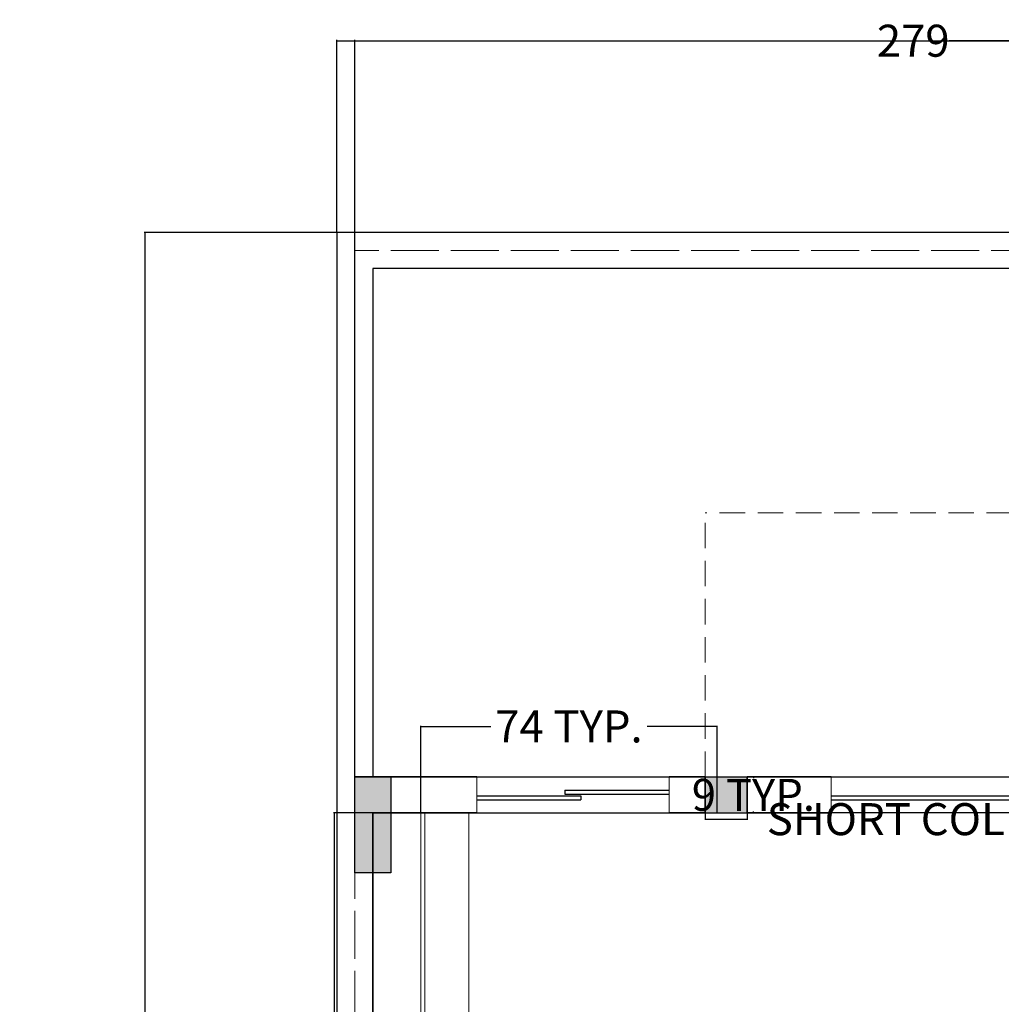
# Model space of a CAD drawing. Units: inches. Extents: x -48 to 50072, y 0 to 21068.
# Tile 67 of 75: x 680 to 925, y 1049 to 1295. Entities that reach past the tile are written whole.
import ezdxf

# ---------------------------------------------------------------- set-up
doc = ezdxf.new("R2010")
doc.units = ezdxf.units.IN
doc.header["$MEASUREMENT"] = 0
doc.linetypes.add('ACAD_ISO02W100', pattern=[15, 12, -3])
doc.linetypes.add('HIDDEN', pattern=[9.525, 6.35, -3.175])
for name, color, linetype, lineweight in [('A-ANNO-DIMS', 2, 'Continuous', 18), ('A-COLS', 1, 'Continuous', 35), ('A-DOOR', 4, 'Continuous', 18), ('A-FLOR-CASE', 9, 'Continuous', 18), ('A-FLOR-OVHD', 8, 'HIDDEN', 13), ('A-GLAZ', 4, 'Continuous', 18), ('A-WALL', 7, 'Continuous', 35), ('C-PROP', 7, 'Continuous', 25), ('C-PROP-REF', 32, 'ACAD_ISO02W100', 13)]:
    doc.layers.add(name, color=color, linetype=linetype, lineweight=lineweight)
doc.layers.add('Layer3', color=176, linetype='Continuous')
doc.styles.get("Standard").update_dxf_attribs({"font": 'arial.ttf'})
doc.dimstyles.get("Standard").update_dxf_attribs({"dimtxt": 8, "dimasz": 0.18, "dimexe": 0.18, "dimexo": 0.0625, "dimgap": 0.09, "dimtad": 0, "dimtih": 1, "dimtoh": 1, "dimdec": 1, "dimzin": 0, "dimdsep": 46, "dimlunit": 4, "dimtxsty": 'Standard', "dimblk": 'ARCHTICK', "dimcen": 0.09, "dimadec": 0, "dimazin": 0, "dimtfac": 1, "dimtdec": 1, "dimtofl": 0, "dimtmove": 0, "dimatfit": 3, "dimldrblk": 'ARCHTICK', "dimfxl": 1, "dimtolj": 1, "dimtzin": 0, "dimarcsym": 0})

# ---------------------------------------------------------------- blocks, each defined once
blk = doc.blocks.new('khll')
at = {"layer": 'Defpoints'}
h = blk.add_hatch(color=256, dxfattribs=at)
h.dxf.hatch_style = 1
h.paths.add_polyline_path([(105.52, 1025.77), (116.02, 1025.77), (116.02, 1034.77), (105.52, 1034.77)])
for p, q in [((105.52, 1025.77), (105.52, 1034.77)), ((116.02, 1025.77), (116.02, 1034.77))]:
    blk.add_line(p, q)
for p, q in [((105.52, 1034.77), (116.02, 1034.77)), ((105.52, 1025.77), (116.02, 1025.77))]:
    blk.add_line(p, q, dxfattribs=at)
blk = doc.blocks.new('bnniku')
at = {"layer": 'Defpoints'}
h = blk.add_hatch(color=256, dxfattribs=at)
h.dxf.hatch_style = 1
h.paths.add_polyline_path([(767.55, 1114.04), (758.55, 1114.04), (758.55, 1090.04), (767.55, 1090.04)])
for p, q in [((758.55, 1114.04), (767.55, 1114.04)), ((758.55, 1090.04), (758.55, 1114.04)), ((767.55, 1114.04), (767.55, 1090.04)), ((767.55, 1090.04), (758.55, 1090.04))]:
    blk.add_line(p, q, dxfattribs=at)
blk = doc.blocks.new('windom')
for p, q in [((48.52, 1025.77), (48.52, 1034.77)), ((96.52, 1025.77), (96.52, 1034.77))]:
    blk.add_line(p, q)
at = {"layer": 'Defpoints'}
for p, q in [((70.52, 1031.47), (96.52, 1031.47)), ((70.52, 1031.47), (70.52, 1030.47)), ((48.52, 1030.07), (74.52, 1030.07)), ((48.52, 1029.07), (74.52, 1029.07)), ((70.52, 1030.47), (96.52, 1030.47)), ((74.52, 1030.07), (74.52, 1029.07))]:
    blk.add_line(p, q, dxfattribs=at)
at = {"layer": 'Layer3'}
for p, q in [((48.52, 1034.77), (96.52, 1034.77)), ((48.52, 1025.77), (96.52, 1025.77))]:
    blk.add_line(p, q, dxfattribs=at)
blk = doc.blocks.new('sliding')
blk.add_line((137.02, 1025.77), (137.02, 1034.77))
at = {"layer": 'Defpoints'}
for p, q in [((234.12, 1034.77), (234.12, 1025.77)), ((183.57, 1031.47), (234.12, 1031.47)), ((183.57, 1031.47), (183.57, 1030.47)), ((137.02, 1030.07), (187.57, 1030.07)), ((137.02, 1029.07), (187.57, 1029.07)), ((183.57, 1030.47), (234.12, 1030.47)), ((187.57, 1030.07), (187.57, 1029.07))]:
    blk.add_line(p, q, dxfattribs=at)
at = {"layer": 'Layer3'}
for p, q in [((137.02, 1034.77), (234.12, 1034.77)), ((234.12, 1025.77), (137.02, 1025.77))]:
    blk.add_line(p, q, dxfattribs=at)
blk = doc.blocks.new('WARDROBE-L-RETURN')
for p, q in [((0, 144), (0, 0)), ((1, 144), (1, 1)), ((12, 144), (12, 12)), ((74, 12), (12, 12)), ((74, 1), (1, 1)), ((74, 0), (0, 0))]:
    blk.add_line(p, q)
blk = doc.blocks.new('_ArchTick')
at = {"color": 0, "linetype": 'ByBlock', "const_width": 0.15}
blk.add_lwpolyline([(-0.5, -0.5), (0.5, 0.5)], dxfattribs=at)
blk = doc.blocks.new('*D50')
at = {"layer": 'A-ANNO-DIMS', "color": 0, "lineweight": -2, "transparency": 16777216}
for p, q in [((850.76, 1096.4), (850.76, 1094.71)), ((850.76, 1094.89), (861.26, 1094.89)), ((861.26, 1096.4), (861.26, 1094.71)), ((861.26, 1094.89), (861.44, 1094.89))]:
    blk.add_line(p, q, dxfattribs=at)
at = {"layer": 'Defpoints', "color": 0, "transparency": 16777216}
for p in [(850.76, 1096.46), (861.26, 1096.46), (861.26, 1094.89)]:
    blk.add_point(p, dxfattribs=at)
at = {"layer": 'A-ANNO-DIMS', "color": 0, "lineweight": -2, "transparency": 16777216, "xscale": 0.18, "yscale": 0.18, "zscale": 0.18, "rotation": 180}
blk.add_blockref('_ArchTick', (850.76, 1094.89), dxfattribs=at)
at = {"layer": 'A-ANNO-DIMS', "color": 0, "lineweight": -2, "transparency": 16777216, "xscale": 0.18, "yscale": 0.18, "zscale": 0.18}
blk.add_blockref('_ArchTick', (861.26, 1094.89), dxfattribs=at)
at = {"layer": 'A-ANNO-DIMS', "color": 0, "transparency": 16777216, "insert": (927.86, 1094.89), "char_height": 8, "attachment_point": 5}
blk.add_mtext('\\A1;SHORT COLUMN 11 TYP.', dxfattribs=at)
blk = doc.blocks.new('*D51')
at = {"layer": 'A-ANNO-DIMS', "color": 0, "lineweight": -2, "transparency": 16777216}
for p, q in [((861.32, 1105.46), (863.02, 1105.46)), ((862.84, 1105.46), (862.84, 1105.14)), ((861.32, 1096.46), (863.02, 1096.46)), ((862.84, 1096.46), (862.84, 1096.79))]:
    blk.add_line(p, q, dxfattribs=at)
at = {"layer": 'Defpoints', "color": 0, "transparency": 16777216}
for p in [(861.26, 1105.46), (862.84, 1105.46), (861.26, 1096.46)]:
    blk.add_point(p, dxfattribs=at)
at = {"layer": 'A-ANNO-DIMS', "color": 0, "lineweight": -2, "transparency": 16777216, "xscale": 0.18, "yscale": 0.18, "zscale": 0.18}
for p, rotation in [((862.84, 1105.46), 90), ((862.84, 1096.46), 270)]:
    blk.add_blockref('_ArchTick', p, dxfattribs=dict(at, rotation=rotation))
at = {"layer": 'A-ANNO-DIMS', "color": 0, "transparency": 16777216, "insert": (862.84, 1100.96), "char_height": 8, "attachment_point": 5}
blk.add_mtext('\\A1;9 TYP.', dxfattribs=at)
blk = doc.blocks.new('*D102')
at = {"layer": 'A-ANNO-DIMS', "color": 0, "lineweight": -2, "transparency": 16777216}
for p, q in [((779.7, 1096.46), (757.98, 1096.46)), ((758.16, 1096.46), (758.16, 1028.69)), ((758.16, 952.46), (758.16, 1020.23)), ((779.7, 952.46), (757.98, 952.46))]:
    blk.add_line(p, q, dxfattribs=at)
at = {"layer": 'Defpoints', "color": 0, "transparency": 16777216}
for p in [(758.16, 1096.46), (779.76, 1096.46), (779.76, 952.46)]:
    blk.add_point(p, dxfattribs=at)
at = {"layer": 'A-ANNO-DIMS', "color": 0, "lineweight": -2, "transparency": 16777216, "xscale": 0.18, "yscale": 0.18, "zscale": 0.18}
for p, rotation in [((758.16, 1096.46), 90), ((758.16, 952.46), 270)]:
    blk.add_blockref('_ArchTick', p, dxfattribs=dict(at, rotation=rotation))
at = {"layer": 'A-ANNO-DIMS', "color": 0, "transparency": 16777216, "insert": (758.16, 1024.46), "char_height": 8, "attachment_point": 5}
blk.add_mtext('\\A1;L-RETURN WARDROBE 144 TYP.', dxfattribs=at)
blk = doc.blocks.new('*D103')
at = {"layer": 'A-ANNO-DIMS', "color": 0, "lineweight": -2, "transparency": 16777216}
for p, q in [((779.76, 1096.53), (779.76, 1118.24)), ((779.76, 1118.06), (797.23, 1118.06)), ((853.76, 1118.06), (836.29, 1118.06)), ((853.76, 1096.53), (853.76, 1118.24))]:
    blk.add_line(p, q, dxfattribs=at)
at = {"layer": 'Defpoints', "color": 0, "transparency": 16777216}
for p in [(853.76, 1118.06), (779.76, 1096.46), (853.76, 1096.46)]:
    blk.add_point(p, dxfattribs=at)
at = {"layer": 'A-ANNO-DIMS', "color": 0, "lineweight": -2, "transparency": 16777216, "xscale": 0.18, "yscale": 0.18, "zscale": 0.18, "rotation": 180}
blk.add_blockref('_ArchTick', (779.76, 1118.06), dxfattribs=at)
at = {"layer": 'A-ANNO-DIMS', "color": 0, "lineweight": -2, "transparency": 16777216, "xscale": 0.18, "yscale": 0.18, "zscale": 0.18}
blk.add_blockref('_ArchTick', (853.76, 1118.06), dxfattribs=at)
at = {"layer": 'A-ANNO-DIMS', "color": 0, "transparency": 16777216, "insert": (816.76, 1118.06), "char_height": 8, "attachment_point": 5}
blk.add_mtext('\\A1;74 TYP.', dxfattribs=at)
blk = doc.blocks.new('*D129')
at = {"layer": 'A-ANNO-DIMS', "color": 0, "lineweight": -2, "transparency": 16777216}
for p, q in [((758.76, 1241.53), (758.76, 1289.59)), ((758.76, 1289.41), (1019.85, 1289.41)), ((1298.76, 1289.41), (1037.67, 1289.41)), ((1298.76, 1241.53), (1298.76, 1289.59))]:
    blk.add_line(p, q, dxfattribs=at)
at = {"layer": 'Defpoints', "color": 0, "transparency": 16777216}
for p in [(1298.76, 1289.41), (758.76, 1241.46), (1298.76, 1241.46)]:
    blk.add_point(p, dxfattribs=at)
at = {"layer": 'A-ANNO-DIMS', "color": 0, "lineweight": -2, "transparency": 16777216, "xscale": 0.18, "yscale": 0.18, "zscale": 0.18, "rotation": 180}
blk.add_blockref('_ArchTick', (758.76, 1289.41), dxfattribs=at)
at = {"layer": 'A-ANNO-DIMS', "color": 0, "lineweight": -2, "transparency": 16777216, "xscale": 0.18, "yscale": 0.18, "zscale": 0.18}
blk.add_blockref('_ArchTick', (1298.76, 1289.41), dxfattribs=at)
at = {"layer": 'A-ANNO-DIMS', "color": 0, "transparency": 16777216, "insert": (1028.76, 1289.41), "char_height": 8, "attachment_point": 5}
blk.add_mtext('\\A1;540', dxfattribs=at)
blk = doc.blocks.new('*D130')
at = {"layer": 'A-ANNO-DIMS', "color": 0, "lineweight": -2, "transparency": 16777216}
for p, q in [((758.7, 1241.46), (710.63, 1241.46)), ((710.81, 1241.46), (710.81, 767.29)), ((710.81, 284.76), (710.81, 758.94)), ((758.7, 284.76), (710.63, 284.76))]:
    blk.add_line(p, q, dxfattribs=at)
at = {"layer": 'Defpoints', "color": 0, "transparency": 16777216}
for p in [(710.81, 1241.46), (758.76, 1241.46), (758.76, 284.76)]:
    blk.add_point(p, dxfattribs=at)
at = {"layer": 'A-ANNO-DIMS', "color": 0, "lineweight": -2, "transparency": 16777216, "xscale": 0.18, "yscale": 0.18, "zscale": 0.18}
for p, rotation in [((710.81, 1241.46), 90), ((710.81, 284.76), 270)]:
    blk.add_blockref('_ArchTick', p, dxfattribs=dict(at, rotation=rotation))
at = {"layer": 'A-ANNO-DIMS', "color": 0, "transparency": 16777216, "insert": (710.81, 763.11), "char_height": 8, "attachment_point": 5}
blk.add_mtext('\\A1;956.7', dxfattribs=at)
blk = doc.blocks.new('*D142')
at = {"layer": 'A-ANNO-DIMS', "color": 0, "lineweight": -2, "transparency": 16777216}
for p, q in [((763.26, 1105.53), (763.26, 1289.59)), ((763.26, 1289.41), (893.76, 1289.41)), ((1042.26, 1289.41), (911.76, 1289.41)), ((1042.26, 1105.53), (1042.26, 1289.59))]:
    blk.add_line(p, q, dxfattribs=at)
at = {"layer": 'Defpoints', "color": 0, "transparency": 16777216}
for p in [(1042.26, 1289.41), (763.26, 1105.46), (1042.26, 1105.46)]:
    blk.add_point(p, dxfattribs=at)
at = {"layer": 'A-ANNO-DIMS', "color": 0, "lineweight": -2, "transparency": 16777216, "xscale": 0.18, "yscale": 0.18, "zscale": 0.18, "rotation": 180}
blk.add_blockref('_ArchTick', (763.26, 1289.41), dxfattribs=at)
at = {"layer": 'A-ANNO-DIMS', "color": 0, "lineweight": -2, "transparency": 16777216, "xscale": 0.18, "yscale": 0.18, "zscale": 0.18}
blk.add_blockref('_ArchTick', (1042.26, 1289.41), dxfattribs=at)
at = {"layer": 'A-ANNO-DIMS', "color": 0, "transparency": 16777216, "insert": (902.76, 1289.41), "char_height": 8, "attachment_point": 5}
blk.add_mtext('\\A1;279', dxfattribs=at)

msp = doc.modelspace()

# ---------------------------------------------------------------- linework, layer by layer
at = {"layer": 'A-FLOR-OVHD'}
for p in [(850.761, 1105.464), (1051.261, 1171.464)]:
    msp.add_line(p, (850.761, 1171.464), dxfattribs=at)
at = {"layer": 'A-WALL'}
for p, q in [((793.761, 1105.464), (763.261, 1105.464)), ((850.761, 1105.464), (841.761, 1105.464)), ((882.261, 1105.464), (861.261, 1105.464)), ((793.761, 1096.464), (767.761, 1096.464)), ((767.761, 1096.464), (767.761, 940.464)), ((850.761, 1096.464), (841.761, 1096.464)), ((882.261, 1096.464), (861.261, 1096.464))]:
    msp.add_line(p, q, dxfattribs=at)
at = {"layer": 'C-PROP'}
for p, q in [((1298.761, 1241.464), (758.761, 1241.464)), ((758.761, 1241.464), (758.761, 284.764)), ((1289.761, 1232.464), (767.761, 1232.464)), ((767.761, 1232.464), (767.761, 1105.464))]:
    msp.add_line(p, q, dxfattribs=at)
at = {"layer": 'C-PROP-REF'}
for p, q in [((1294.261, 1236.964), (763.261, 1236.964)), ((763.261, 1236.964), (763.261, 284.764))]:
    msp.add_line(p, q, dxfattribs=at)

# ---------------------------------------------------------------- block references
at = {"layer": 'A-COLS'}
for name, p in [('bnniku', (4.709, -8.573)), ('khll', (745.244, 70.689))]:
    msp.add_blockref(name, p, dxfattribs=at)
at = {"layer": 'A-DOOR'}
msp.add_blockref('sliding', (745.244, 70.689), dxfattribs=at)
at = {"layer": 'A-FLOR-CASE'}
msp.add_blockref('WARDROBE-L-RETURN', (779.761, 952.464), dxfattribs=at)
at = {"layer": 'A-GLAZ'}
msp.add_blockref('windom', (745.244, 70.689), dxfattribs=at)

# ---------------------------------------------------------------- dimensions: what is measured, and where the dimension line sits
at = {"layer": 'A-ANNO-DIMS'}
for base, p1, p2, picture, middle in [((1298.761, 1289.414), (758.761, 1241.464), (1298.761, 1241.464), '*D129', (1028.761, 1289.414)), ((1042.261, 1289.414), (763.261, 1105.464), (1042.261, 1105.464), '*D142', (902.761, 1289.414))]:
    dim = msp.add_linear_dim(base=base, p1=p1, p2=p2, dimstyle='Standard', override={"dimdec": 0, "dimlfac": 1, "dimrnd": 0, "dimzin": 0, "dimdsep": 46, "dimlunit": 2}, dxfattribs=at)
    dim.commit()
    dim.dimension.update_dxf_attribs({"geometry": picture, "text_midpoint": middle})
dim = msp.add_linear_dim(base=(710.811, 1241.464), p1=(758.761, 284.764), p2=(758.761, 1241.464), angle=90, dimstyle='Standard', override={"dimdec": 1, "dimlfac": 1, "dimrnd": 0, "dimzin": 0, "dimdsep": 46, "dimlunit": 2}, dxfattribs=at)
dim.commit()
dim.dimension.update_dxf_attribs({"geometry": '*D130', "text_midpoint": (710.811, 763.114)})
for base, p1, p2, text, picture, middle in [((853.761, 1118.064), (779.761, 1096.464), (853.761, 1096.464), '<> TYP.', '*D103', (816.761, 1118.064)), ((861.260753509, 1094.889050042), (850.760753509, 1096.464050042), (861.260753509, 1096.464050042), 'SHORT COLUMN <> TYP.', '*D50', (927.860903577, 1094.889050042))]:
    dim = msp.add_linear_dim(base=base, p1=p1, p2=p2, text=text, dimstyle='Standard', override={"dimdec": 0, "dimlfac": 1, "dimrnd": 0, "dimzin": 0, "dimdsep": 46, "dimlunit": 2}, dxfattribs=at)
    dim.commit()
    dim.dimension.update_dxf_attribs({"geometry": picture, "text_midpoint": middle})
for base, p1, p2, text, picture, middle in [((862.836, 1105.464), (861.261, 1096.464), (861.261, 1105.464), '<> TYP.', '*D51', (862.836, 1100.964)), ((758.161, 1096.464), (779.761, 952.464), (779.761, 1096.464), 'L-RETURN WARDROBE <> TYP.', '*D102', (758.161, 1024.464))]:
    dim = msp.add_linear_dim(base=base, p1=p1, p2=p2, angle=90, text=text, dimstyle='Standard', override={"dimdec": 0, "dimlfac": 1, "dimrnd": 0, "dimzin": 0, "dimdsep": 46, "dimlunit": 2}, dxfattribs=at)
    dim.commit()
    dim.dimension.update_dxf_attribs({"geometry": picture, "text_midpoint": middle})

doc.saveas('drawing.dxf')
